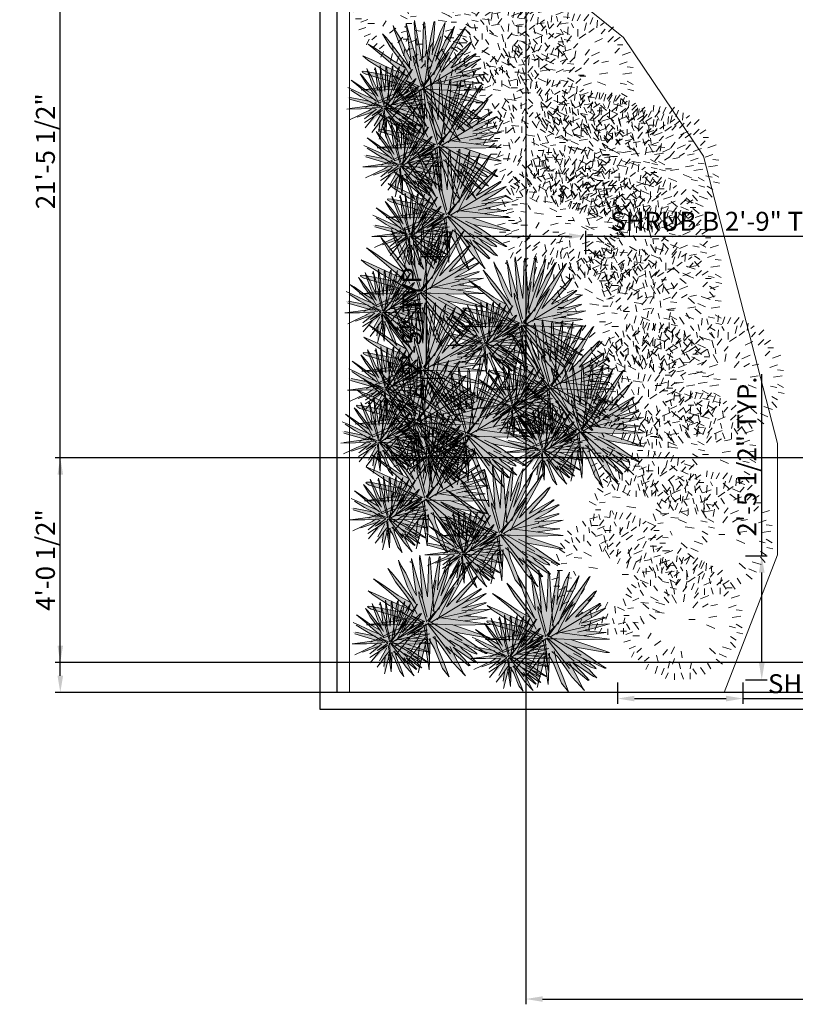
# Model space of a CAD drawing. Units: inches. Extents: x 1239 to 2276906, y 2273 to 321338.
# Tile 1 of 23: x 1239 to 1424, y 2276 to 2510. Entities that reach past the tile are written whole.
import ezdxf

# ---------------------------------------------------------------- set-up
doc = ezdxf.new("R2010")
doc.units = ezdxf.units.IN
for name, color, linetype, lineweight in [('A-ANNO-DIMS', 2, 'Continuous', 18), ('C-PROP', 7, 'Continuous', 25), ('L-PLNT', 94, 'Continuous', 13)]:
    doc.layers.add(name, color=color, linetype=linetype, lineweight=lineweight)
doc.styles.get("Standard").update_dxf_attribs({"font": 'arial.ttf'})
doc.dimstyles.new('ISO-25', dxfattribs={"dimtxt": 4.5, "dimasz": 4, "dimexe": 1.25, "dimexo": 0.625, "dimtad": 1, "dimdec": 1, "dimlunit": 3, "dimtxsty": 'Standard', "dimcen": 2.5, "dimadec": 0, "dimazin": 0, "dimtfac": 1, "dimtdec": 1, "dimtmove": 0, "dimatfit": 3, "dimfxl": 1, "dimarcsym": 0})

# ---------------------------------------------------------------- blocks, each defined once
blk = doc.blocks.new('A$C20C17E7E')
for p, q in [((1.899, 5.117), (1.929, 5.423)), ((2.205, 5.147), (2.144, 5.393)), ((2.635, 5.271), (2.665, 5.546)), ((2.849, 5.179), (2.941, 5.485)), ((3.063, 5.179), (3.217, 5.455)), ((3.37, 5.179), (3.584, 5.455)), ((3.646, 5.025), (3.768, 5.332)), ((1.195, 4.597), (1.134, 4.871)), ((1.562, 4.871), (1.409, 5.086)), ((1.807, 4.871), (1.746, 5.147)), ((2.174, 4.903), (2.359, 5.147)), ((2.635, 4.565), (2.665, 4.903)), ((2.91, 4.871), (2.819, 5.056)), ((3.401, 4.749), (3.492, 5.086)), ((3.952, 4.871), (3.983, 5.21)), ((4.105, 4.964), (4.259, 5.086)), ((4.472, 4.688), (4.687, 4.903)), ((0.919, 4.474), (0.735, 4.658)), ((1.47, 4.198), (1.47, 4.474)), ((1.716, 4.565), (1.685, 4.81)), ((1.991, 4.443), (1.807, 4.627)), ((2.45, 4.565), (2.328, 4.81)), ((2.45, 4.106), (2.359, 4.443)), ((2.604, 4.228), (2.819, 4.504)), ((3.095, 4.474), (3.095, 4.81)), ((3.156, 4.382), (3.462, 4.597)), ((3.584, 4.658), (3.829, 4.841)), ((4.135, 4.597), (4.32, 4.81)), ((4.442, 4.228), (4.687, 4.474)), ((4.717, 4.259), (4.993, 4.443)), ((0.613, 3.861), (0.428, 4.106)), ((0.827, 4.106), (0.613, 4.259)), ((0.98, 4.137), (0.919, 4.352)), ((1.164, 3.77), (1.01, 4.014)), ((1.286, 4.137), (1.102, 4.352)), ((1.777, 3.983), (1.623, 4.198)), ((2.267, 3.739), (2.174, 4.045)), ((2.543, 3.831), (2.513, 4.076)), ((2.91, 3.953), (3.095, 4.167)), ((3.86, 4.228), (4.196, 4.382)), ((4.871, 4.106), (5.117, 4.106)), ((0.367, 3.31), (0.244, 3.616)), ((0.613, 3.677), (0.367, 3.831)), ((0.949, 3.646), (0.674, 3.524)), ((1.807, 3.524), (1.47, 3.707)), ((2.635, 3.431), (2.42, 3.8)), ((2.941, 3.494), (3.002, 3.831)), ((3.431, 3.646), (3.614, 3.892)), ((3.707, 3.616), (4.074, 3.77)), ((4.748, 3.739), (4.963, 3.953)), ((5.086, 3.646), (5.453, 3.77)), ((0.306, 3.095), (0, 3.249)), ((0.704, 3.218), (0.459, 3.188)), ((1.378, 3.431), (1.041, 3.463)), ((3.37, 3.218), (3.584, 3.494)), ((3.799, 3.249), (4.044, 3.401)), ((4.166, 3.31), (4.472, 3.37)), ((4.963, 3.218), (5.3, 3.34)), ((5.3, 3.125), (5.575, 3.095)), ((0.52, 2.88), (0.276, 2.88)), ((1.102, 2.666), (1.01, 2.849)), ((2.083, 2.973), (1.685, 3.034)), ((3.186, 2.697), (3.462, 2.697)), ((4.074, 2.788), (4.442, 2.849)), ((5.117, 2.788), (5.514, 2.849)), ((0.367, 2.574), (0.03, 2.482)), ((0.919, 2.543), (0.674, 2.574)), ((3.983, 2.452), (4.35, 2.298)), ((4.993, 2.391), (5.269, 2.33)), ((5.3, 2.482), (5.575, 2.33)), ((0.398, 2.176), (0.122, 2.176)), ((0.582, 1.778), (0.276, 1.685)), ((0.674, 2.145), (0.367, 2.022)), ((0.98, 1.961), (0.674, 1.961)), ((1.501, 2.084), (1.347, 1.839)), ((5.056, 1.931), (5.3, 1.778)), ((5.331, 2.115), (5.607, 2.054)), ((0.796, 1.502), (0.52, 1.379)), ((1.071, 1.409), (0.858, 1.226)), ((1.929, 1.748), (1.653, 1.533)), ((2.237, 1.348), (2.022, 1.103)), ((2.543, 1.472), (2.389, 1.164)), ((4.105, 1.409), (4.381, 1.164)), ((4.687, 1.472), (5.086, 1.348)), ((5.056, 1.685), (5.269, 1.44)), ((0.735, 1.257), (0.613, 1.012)), ((1.102, 1.073), (0.919, 0.888)), ((1.409, 1.012), (1.195, 0.827)), ((1.746, 1.103), (1.807, 0.797)), ((2.543, 0.951), (2.45, 0.705)), ((2.849, 1.287), (2.88, 0.981)), ((4.411, 0.92), (4.687, 0.705)), ((4.535, 1.164), (4.871, 1.012)), ((1.378, 0.705), (1.256, 0.46)), ((1.777, 0.614), (1.685, 0.276)), ((2.083, 0.521), (1.961, 0.215)), ((2.328, 0.827), (2.267, 0.521)), ((2.757, 0.736), (2.819, 0.491)), ((3.308, 0.766), (3.247, 0.491)), ((3.37, 0.491), (3.523, 0.245)), ((3.707, 0.552), (3.922, 0.245)), ((4.013, 0.736), (4.166, 0.491)), ((2.267, 0.306), (2.144, 0.062)), ((2.543, 0.276), (2.543, 0)), ((2.849, 0.306), (2.941, 0.03)), ((3.247, 0.306), (3.247, 0.03))]:
    blk.add_line(p, q)
blk = doc.blocks.new('A$C545C060E')
h = blk.add_hatch(color=256)
h.set_gradient(color1=(31, 127, 0), color2=(45, 179, 0), one_color=1, tint=0.35, name='INVSPHERICAL')
h.paths.add_polyline_path([(0.529, 2.393), (0.645, 2.304), (1.889, 1.967), (0.489, 1.77), (1.843, 1.787), (1.618, 1.643), (0.635, 1.178), (1.063, 1.326), (1.966, 1.643), (1.461, 1.231), (1.869, 1.417), (2.379, 1.664), (2.177, 1.5), (1.446, 1.03), (1.981, 1.358), (1.481, 0.744), (2.376, 1.553), (1.986, 0.848), (2.48, 1.336), (1.85, 0.496), (2.266, 0.842), (2.223, 0.533), (2.243, 0.142), (2.487, 1.093), (2.615, 0.257), (2.655, 1.214), (3.074, 0.284), (3.303, 0), (2.908, 1.003), (2.846, 1.271), (2.929, 1.199), (3.853, 0.038), (3.428, 0.832), (3.973, 0.376), (4.009, 0.393), (3.432, 1.008), (3.923, 0.676), (4.175, 0.507), (4.274, 0.474), (4.155, 0.583), (4.009, 0.757), (3.765, 0.932), (3.662, 1.051), (4.067, 0.828), (4.243, 0.779), (4.238, 0.801), (3.802, 1.133), (4.534, 0.795), (4.591, 0.795), (4.42, 0.899), (4.103, 1.12), (3.786, 1.34), (3.464, 1.533), (3.968, 1.441), (4.415, 1.362), (4.571, 1.335), (4.695, 1.33), (3.997, 1.572), (3.423, 1.771), (4.695, 1.782), (3.833, 1.912), (4.591, 2.011), (3.836, 2.079), (4.706, 2.305), (3.951, 2.263), (4.55, 2.506), (4.555, 2.528), (4.493, 2.517), (3.734, 2.332), (4.197, 2.577), (4.56, 2.833), (3.786, 2.523), (4.363, 2.959), (4.394, 2.997), (4.363, 2.997), (3.558, 2.528), (3.549, 2.536), (4.087, 3.155), (4.254, 3.422), (4.191, 3.389), (3.209, 2.381), (4.046, 3.912), (3.999, 3.874), (3.09, 2.626), (3.547, 3.58), (3.666, 3.934), (3.35, 3.438), (3.017, 2.752), (3.225, 3.411), (3.345, 4.064), (3.243, 3.868), (3.184, 3.754), (2.919, 3.073), (2.986, 3.83), (2.991, 4.097), (2.96, 4.075), (2.742, 2.981), (2.732, 2.92), (2.659, 4.026), (2.633, 4.092), (2.612, 4.005), (2.56, 2.719), (2.3, 4.135), (2.382, 2.743), (2.025, 4.026), (2.02, 3.934), (1.968, 3.917), (2.046, 3.874), (2.185, 2.776), (1.976, 3.197), (1.829, 3.524), (1.673, 3.773), (1.577, 3.963), (1.613, 3.821), (1.751, 3.44), (1.89, 3.059), (2.192, 2.446), (1.345, 3.551), (1.215, 3.683), (1.481, 3.234), (2.006, 2.515), (1.567, 2.769), (0.983, 3.176), (0.731, 3.334), (1.255, 2.901), (1.969, 2.294), (0.912, 2.769), (0.549, 2.927), (1.687, 2.199), (0.675, 2.399), (0.554, 2.409)])
h = blk.add_hatch(color=256)
h.set_gradient(color1=(31, 127, 0), color2=(55, 219, 0), one_color=1, tint=0.43, name='SPHERICAL')
h.paths.add_polyline_path([(3.023, 2.188), (3.114, 2.362), (3.471, 3.049), (3.33, 2.866), (2.618, 1.891), (2.679, 1.855), (2.94, 2.013)])
h = blk.add_hatch(color=256)
h.set_gradient(color1=(31, 127, 0), color2=(45, 179, 0), one_color=1, tint=0.35, name='INVSPHERICAL')
h.paths.add_polyline_path([(0.025, 1.517), (0.098, 1.461), (0.877, 1.25), (0, 1.126), (0.848, 1.137), (0.707, 1.047), (0.092, 0.756), (0.36, 0.848), (0.925, 1.047), (0.609, 0.789), (0.865, 0.905), (1.184, 1.06), (1.058, 0.958), (0.6, 0.663), (0.935, 0.868), (0.622, 0.484), (1.182, 0.99), (0.938, 0.549), (1.247, 0.855), (0.853, 0.328), (1.113, 0.545), (1.086, 0.352), (1.099, 0.106), (1.252, 0.703), (1.332, 0.179), (1.357, 0.779), (1.62, 0.195), (1.763, 0.018), (1.515, 0.646), (1.477, 0.814), (1.529, 0.769), (2.108, 0.042), (1.841, 0.539), (2.183, 0.253), (2.206, 0.264), (1.844, 0.649), (2.152, 0.441), (2.31, 0.335), (2.371, 0.315), (2.297, 0.383), (2.206, 0.492), (2.053, 0.602), (1.988, 0.676), (2.242, 0.537), (2.352, 0.506), (2.349, 0.52), (2.076, 0.728), (2.534, 0.516), (2.57, 0.516), (2.463, 0.581), (2.264, 0.719), (2.066, 0.857), (1.864, 0.978), (2.18, 0.921), (2.46, 0.871), (2.557, 0.854), (2.636, 0.851), (2.198, 1.003), (1.839, 1.127), (2.636, 1.134), (2.095, 1.216), (2.57, 1.277), (2.097, 1.32), (2.642, 1.462), (2.169, 1.435), (2.544, 1.588), (2.548, 1.602), (2.509, 1.595), (2.033, 1.479), (2.323, 1.632), (2.551, 1.793), (2.066, 1.598), (2.427, 1.871), (2.447, 1.895), (2.427, 1.895), (1.923, 1.602), (1.917, 1.606), (2.255, 1.994), (2.359, 2.161), (2.32, 2.141), (1.704, 1.509), (2.229, 2.469), (2.199, 2.445), (1.63, 1.663), (1.916, 2.26), (1.991, 2.482), (1.792, 2.172), (1.584, 1.741), (1.714, 2.155), (1.789, 2.564), (1.726, 2.441), (1.688, 2.369), (1.522, 1.943), (1.565, 2.417), (1.568, 2.584), (1.548, 2.571), (1.412, 1.885), (1.405, 1.847), (1.36, 2.54), (1.343, 2.581), (1.33, 2.526), (1.298, 1.721), (1.135, 2.608), (1.186, 1.736), (0.962, 2.54), (0.959, 2.482), (0.927, 2.472), (0.976, 2.445), (1.063, 1.757), (0.932, 2.02), (0.84, 2.226), (0.742, 2.381), (0.682, 2.501), (0.704, 2.411), (0.791, 2.173), (0.878, 1.934), (1.067, 1.55), (0.537, 2.242), (0.455, 2.325), (0.622, 2.044), (0.951, 1.593), (0.676, 1.752), (0.31, 2.007), (0.152, 2.107), (0.48, 1.835), (0.927, 1.455), (0.265, 1.752), (0.038, 1.851), (0.751, 1.395), (0.117, 1.52), (0.041, 1.527)])
h = blk.add_hatch(color=256)
h.set_gradient(color1=(31, 127, 0), color2=(55, 219, 0), one_color=1, tint=0.43, name='SPHERICAL')
h.paths.add_polyline_path([(1.334, 1.202), (1.372, 1.18), (1.536, 1.279), (1.588, 1.388), (1.645, 1.497), (1.868, 1.928), (1.78, 1.813)])
for p, q in [((2.02, 3.934, -52.769), (2.025, 4.026, -52.769)), ((2.025, 4.026, -52.769), (2.389, 2.719, -52.769)), ((2.295, 4.037, -52.769), (2.3, 4.135, -52.769)), ((2.389, 2.643, -52.769), (2.295, 4.037, -52.769)), ((2.3, 4.135, -52.769), (2.534, 2.893, -52.769)), ((2.612, 4.005, -52.769), (2.633, 4.092, -52.769)), ((2.633, 4.092, -52.769), (2.659, 4.026, -52.769)), ((2.659, 4.026, -52.769), (2.732, 2.92, -52.769)), ((2.945, 4.01, -52.769), (2.96, 4.075, -52.769)), ((2.96, 4.075, -52.769), (2.991, 4.097, -52.769)), ((2.991, 4.097, -52.769), (2.986, 3.83, -52.769)), ((3.345, 4.064, -52.769), (3.225, 3.411, -52.769)), ((3.303, 3.983, -52.769), (3.345, 4.064, -52.769)), ((1.215, 3.683, -52.769), (1.481, 3.234, -52.769)), ((1.345, 3.551, -52.769), (1.215, 3.683, -52.769)), ((1.577, 3.963, -52.769), (1.613, 3.821, -52.769)), ((1.673, 3.773, -52.769), (1.577, 3.963, -52.769)), ((1.613, 3.821, -52.769), (1.89, 3.059, -52.769)), ((1.829, 3.524, -52.769), (1.673, 3.773, -52.769)), ((1.968, 3.917, -52.769), (2.02, 3.934, -52.769)), ((2.046, 3.874, -52.769), (1.968, 3.917, -52.769)), ((2.103, 3.378, -52.769), (2.046, 3.874, -52.769)), ((2.591, 3.329, -52.769), (2.612, 4.005, -52.769)), ((2.742, 2.981, -52.769), (2.945, 4.01, -52.769)), ((2.986, 3.83, -52.769), (2.908, 2.964, -52.769)), ((3.095, 3.498, -52.769), (3.184, 3.754, -52.769)), ((3.184, 3.754, -52.769), (3.303, 3.983, -52.769)), ((3.428, 3.553, -52.769), (3.666, 3.934, -52.769)), ((3.508, 3.479, -52.769), (3.625, 3.884, -52.769)), ((3.666, 3.934, -52.769), (3.547, 3.58, -52.769)), ((3.558, 3.269, -52.769), (3.999, 3.874, -52.769)), ((4.046, 3.912, -52.769), (3.635, 3.155, -52.769)), ((3.999, 3.874, -52.769), (4.046, 3.912, -52.769)), ((1.602, 3.229, -52.769), (1.345, 3.551, -52.769)), ((1.976, 3.197, -52.769), (1.829, 3.524, -52.769)), ((2.186, 2.773, -52.769), (2.103, 3.378, -52.769)), ((3.198, 3.588, -52.769), (2.75, 2.248, -52.769)), ((2.919, 3.073, -52.769), (3.095, 3.498, -52.769)), ((3.225, 3.411, -52.769), (3.017, 2.752, -52.769)), ((3.547, 3.58, -52.769), (3.085, 2.626, -52.769)), ((3.298, 3.329, -52.769), (3.35, 3.438, -52.769)), ((3.35, 3.438, -52.769), (3.428, 3.553, -52.769)), ((3.771, 2.975, -52.769), (4.191, 3.389, -52.769)), ((4.254, 3.422, -52.769), (4.087, 3.155, -52.769)), ((4.191, 3.389, -52.769), (4.254, 3.422, -52.769)), ((0.731, 3.334, -52.769), (1.255, 2.901, -52.769)), ((0.983, 3.176, -52.769), (0.731, 3.334, -52.769)), ((1.567, 2.769, -52.769), (0.983, 3.176, -52.769)), ((1.481, 3.234, -52.769), (1.819, 2.785, -52.769)), ((2.157, 2.505, -52.769), (1.602, 3.229, -52.769)), ((1.89, 3.059, -52.769), (2.192, 2.446, -52.769)), ((2.102, 2.927, -52.769), (1.976, 3.197, -52.769)), ((2.56, 2.719, -52.769), (2.591, 3.329, -52.769)), ((2.849, 3.284, -52.769), (2.65, 1.996, -52.769)), ((3.017, 2.752, -52.769), (3.298, 3.329, -52.769)), ((3.09, 2.626, -52.769), (3.558, 3.269, -52.769)), ((3.471, 3.049, -52.769), (3.114, 2.362, -52.769)), ((3.635, 3.155, -52.769), (3.209, 2.381, -52.769)), ((3.33, 2.866, -52.769), (3.471, 3.049, -52.769)), ((4.087, 3.155, -52.769), (3.542, 2.528, -52.769)), ((0.549, 2.927, -52.769), (0.72, 2.785, -52.769)), ((0.912, 2.769, -52.769), (0.549, 2.927, -52.769)), ((0.72, 2.785, -52.769), (1.27, 2.43, -52.769)), ((1.522, 2.483, -52.769), (0.912, 2.769, -52.769)), ((1.255, 2.901, -52.769), (1.653, 2.552, -52.769)), ((2.006, 2.515, -52.769), (1.567, 2.769, -52.769)), ((1.819, 2.785, -52.769), (2.016, 2.494, -52.769)), ((2.192, 2.764, -52.769), (2.102, 2.927, -52.769)), ((2.269, 2.899, -52.769), (2.394, 2.654, -52.769)), ((2.279, 2.724, -52.769), (2.269, 2.899, -52.769)), ((2.539, 1.864, -52.769), (2.279, 2.724, -52.769)), ((2.534, 2.893, -52.769), (2.56, 2.719, -52.769)), ((2.6, 1.866, -52.769), (3.33, 2.866, -52.769)), ((2.732, 2.92, -52.769), (2.783, 2.212, -52.769)), ((3.209, 2.381, -52.769), (3.771, 2.975, -52.769)), ((3.558, 2.528, -52.769), (4.327, 2.975, -52.769)), ((4.363, 2.959, -52.769), (3.786, 2.523, -52.769)), ((3.797, 2.528, -52.769), (4.191, 2.692, -52.769)), ((4.191, 2.692, -52.769), (4.514, 2.822, -52.769)), ((4.56, 2.833, -52.769), (4.197, 2.577, -52.769)), ((4.327, 2.975, -52.769), (4.363, 2.997, -52.769)), ((4.394, 2.997, -52.769), (4.363, 2.959, -52.769)), ((4.363, 2.997, -52.769), (4.394, 2.997, -52.769)), ((4.514, 2.822, -52.769), (4.56, 2.833, -52.769)), ((0.554, 2.409, -52.769), (0.529, 2.393, -52.769)), ((0.529, 2.393, -52.769), (0.539, 2.367, -52.769)), ((0.539, 2.367, -52.769), (0.645, 2.304, -52.769)), ((0.675, 2.399, -52.769), (0.554, 2.409, -52.769)), ((1.32, 2.272, -52.769), (0.675, 2.399, -52.769)), ((0.682, 2.501), (0.704, 2.411)), ((0.742, 2.381), (0.682, 2.501)), ((0.704, 2.411), (0.878, 1.934)), ((0.84, 2.226), (0.742, 2.381)), ((0.927, 2.472), (0.959, 2.482)), ((0.976, 2.445), (0.927, 2.472)), ((0.959, 2.482), (0.962, 2.54)), ((0.962, 2.54), (1.19, 1.721)), ((1.011, 2.134), (0.976, 2.445)), ((1.132, 2.547), (1.135, 2.608)), ((1.19, 1.673), (1.132, 2.547)), ((1.135, 2.608), (1.281, 1.83)), ((1.27, 2.43, -52.769), (1.764, 2.156, -52.769)), ((1.317, 2.103), (1.33, 2.526)), ((1.33, 2.526), (1.343, 2.581)), ((1.343, 2.581), (1.36, 2.54)), ((1.36, 2.54), (1.405, 1.847)), ((1.412, 1.885), (1.539, 2.53)), ((1.565, 2.417), (1.516, 1.875)), ((2.046, 2.261, -52.769), (1.522, 2.483, -52.769)), ((1.539, 2.53), (1.548, 2.571)), ((1.548, 2.571), (1.568, 2.584)), ((1.568, 2.584), (1.565, 2.417)), ((1.633, 2.209), (1.688, 2.369)), ((1.653, 2.552, -52.769), (2.087, 2.198, -52.769)), ((1.688, 2.369), (1.763, 2.513)), ((1.789, 2.564), (1.714, 2.155)), ((1.763, 2.513), (1.789, 2.564)), ((1.841, 2.243), (1.991, 2.482)), ((1.891, 2.197), (1.965, 2.451)), ((1.991, 2.482), (1.916, 2.26)), ((1.923, 2.066), (2.199, 2.445)), ((2.229, 2.469), (1.971, 1.994)), ((2.016, 2.494, -52.769), (2.208, 2.129, -52.769)), ((2.199, 2.445), (2.229, 2.469)), ((2.394, 2.654, -52.769), (2.55, 2.027, -52.769)), ((3.786, 2.523, -52.769), (2.674, 1.853, -52.769)), ((3.085, 2.626, -52.769), (2.955, 2.288, -52.769)), ((3.114, 2.362, -52.769), (3.023, 2.188, -52.769)), ((3.734, 2.332, -52.769), (4.493, 2.517, -52.769)), ((3.848, 2.381, -52.769), (3.734, 2.332, -52.769)), ((4.197, 2.577, -52.769), (3.848, 2.381, -52.769)), ((4.55, 2.506, -52.769), (3.854, 2.223, -52.769)), ((4.493, 2.517, -52.769), (4.555, 2.528, -52.769)), ((4.555, 2.528, -52.769), (4.55, 2.506, -52.769)), ((0.152, 2.107), (0.48, 1.835)), ((0.31, 2.007), (0.152, 2.107)), ((0.676, 1.752), (0.31, 2.007)), ((0.455, 2.325), (0.622, 2.044)), ((0.537, 2.242), (0.455, 2.325)), ((0.698, 2.04), (0.537, 2.242)), ((0.622, 2.044), (0.834, 1.762)), ((0.645, 2.304, -52.769), (1.734, 1.992, -52.769)), ((1.045, 1.587), (0.698, 2.04)), ((0.932, 2.02), (0.84, 2.226)), ((1.011, 1.851), (0.932, 2.02)), ((1.063, 1.755), (1.011, 2.134)), ((1.298, 1.721), (1.317, 2.103)), ((1.769, 2.182, -52.769), (1.32, 2.272, -52.769)), ((1.479, 2.075), (1.354, 1.268)), ((1.697, 2.266), (1.416, 1.426)), ((1.522, 1.943), (1.633, 2.209)), ((1.714, 2.155), (1.584, 1.741)), ((1.584, 1.741), (1.76, 2.103)), ((1.916, 2.26), (1.627, 1.663)), ((1.63, 1.663), (1.923, 2.066)), ((1.76, 2.103), (1.792, 2.172)), ((1.764, 2.156, -52.769), (2.182, 1.902, -52.769)), ((1.792, 2.172), (1.841, 2.243)), ((2.009, 2.092, -52.769), (2.476, 1.885, -52.769)), ((2.425, 1.814, -52.769), (2.009, 2.092, -52.769)), ((2.056, 1.881), (2.32, 2.141)), ((2.359, 2.161), (2.255, 1.994)), ((2.32, 2.141), (2.359, 2.161)), ((2.565, 1.907, -52.769), (2.84, 2.229, -52.769)), ((2.84, 2.229, -52.769), (2.606, 1.885, -52.769)), ((3.878, 2.205, -52.769), (2.857, 1.97, -52.769)), ((3.023, 2.188, -52.769), (2.907, 1.944, -52.769)), ((4.228, 2.169, -52.769), (3.61, 2.027, -52.769)), ((3.734, 2.25, -52.769), (4.301, 2.283, -52.769)), ((3.807, 2.082, -52.769), (4.264, 2.038, -52.769)), ((4.591, 2.011, -52.769), (3.833, 1.912, -52.769)), ((3.886, 2.102, -52.769), (3.98, 2.099, -52.769)), ((3.949, 2.282, -52.769), (4.001, 2.285, -52.769)), ((3.98, 2.099, -52.769), (4.025, 2.091, -52.769)), ((4.001, 2.285, -52.769), (4.042, 2.282, -52.769)), ((4.706, 2.305, -52.769), (4.228, 2.169, -52.769)), ((4.264, 2.038, -52.769), (4.534, 2.016, -52.769)), ((4.301, 2.283, -52.769), (4.706, 2.305, -52.769)), ((4.534, 2.016, -52.769), (4.591, 2.011, -52.769)), ((0.265, 1.752), (0.038, 1.851)), ((0.145, 1.762), (0.49, 1.54)), ((0.647, 1.573), (0.265, 1.752)), ((0.48, 1.835), (0.729, 1.617)), ((0.64, 1.791, -52.769), (0.489, 1.77, -52.769)), ((0.489, 1.77, -52.769), (1.275, 1.775, -52.769)), ((1.068, 1.844, -52.769), (0.64, 1.791, -52.769)), ((0.951, 1.593), (0.676, 1.752)), ((0.834, 1.762), (0.957, 1.58)), ((0.878, 1.934), (1.067, 1.55)), ((1.067, 1.749), (1.011, 1.851)), ((1.981, 1.981, -52.769), (1.068, 1.844, -52.769)), ((1.115, 1.834), (1.194, 1.68)), ((1.122, 1.724), (1.115, 1.834)), ((1.285, 1.185), (1.122, 1.724)), ((1.194, 1.68), (1.291, 1.288)), ((1.275, 1.775, -52.769), (2.051, 1.791, -52.769)), ((1.281, 1.83), (1.298, 1.721)), ((1.323, 1.186), (1.78, 1.813)), ((1.405, 1.847), (1.438, 1.404)), ((1.678, 1.675, -52.769), (1.618, 1.643, -52.769)), ((1.868, 1.928), (1.645, 1.497)), ((1.865, 1.801, -52.769), (1.678, 1.675, -52.769)), ((1.971, 1.994), (1.704, 1.509)), ((1.704, 1.509), (2.056, 1.881)), ((1.734, 1.992, -52.769), (2.006, 1.949, -52.769)), ((1.78, 1.813), (1.868, 1.928)), ((1.869, 1.417, -52.769), (2.425, 1.814, -52.769)), ((2.456, 1.716, -52.769), (1.869, 1.417, -52.769)), ((1.87, 1.874, -52.769), (2.276, 1.84, -52.769)), ((2.255, 1.994), (1.913, 1.602)), ((1.923, 1.602), (2.404, 1.881)), ((1.966, 1.643, -52.769), (2.107, 1.77, -52.769)), ((2.427, 1.871), (2.066, 1.598)), ((2.072, 1.602), (2.32, 1.704)), ((2.32, 1.704), (2.522, 1.786)), ((2.551, 1.793), (2.323, 1.632)), ((2.404, 1.881), (2.427, 1.895)), ((2.447, 1.895), (2.427, 1.871)), ((2.427, 1.895), (2.447, 1.895)), ((2.617, 0.725, -52.769), (2.456, 1.716, -52.769)), ((2.513, 1.809, -52.769), (2.617, 0.725, -52.769)), ((2.522, 1.786), (2.551, 1.793)), ((2.913, 1.793, -52.769), (2.555, 1.798, -52.769)), ((3.347, 0.787, -52.769), (2.559, 1.822, -52.769)), ((3.504, 1.039, -52.769), (2.584, 1.831, -52.769)), ((3.737, 1.239, -52.769), (2.617, 1.892, -52.769)), ((3.672, 1.76, -52.769), (2.913, 1.793, -52.769)), ((3.516, 1.945, -52.769), (3.028, 2.005, -52.769)), ((3.422, 1.766, -52.769), (4.571, 1.379, -52.769)), ((4.701, 1.782, -52.769), (3.516, 1.945, -52.769)), ((4.695, 1.782, -52.769), (3.672, 1.76, -52.769)), ((0.098, 1.461), (0.78, 1.265)), ((0.521, 1.441), (0.117, 1.52)), ((0.49, 1.54), (0.799, 1.368)), ((0.802, 1.385), (0.521, 1.441)), ((1.048, 1.379, -52.769), (0.635, 1.178, -52.769)), ((0.976, 1.434), (0.647, 1.573)), ((0.729, 1.617), (1.001, 1.395)), ((0.799, 1.368), (1.061, 1.209)), ((0.957, 1.58), (1.077, 1.352)), ((1.345, 1.521, -52.769), (1.048, 1.379, -52.769)), ((1.063, 1.326, -52.769), (1.608, 1.516, -52.769)), ((1.301, 1.212), (1.473, 1.414)), ((1.473, 1.414), (1.327, 1.199)), ((1.618, 1.643, -52.769), (1.345, 1.521, -52.769)), ((2.066, 1.598), (1.369, 1.178)), ((1.446, 1.03, -52.769), (2.177, 1.5, -52.769)), ((1.966, 1.643, -52.769), (1.461, 1.231, -52.769)), ((1.981, 1.358, -52.769), (1.481, 0.744, -52.769)), ((2.123, 1.399), (1.484, 1.252)), ((1.588, 1.388), (1.515, 1.235)), ((1.627, 1.663), (1.545, 1.451)), ((1.645, 1.497), (1.588, 1.388)), ((1.608, 1.516, -52.769), (1.966, 1.643, -52.769)), ((2.343, 1.376), (1.955, 1.288)), ((1.986, 0.848, -52.769), (2.376, 1.553, -52.769)), ((2.033, 1.479), (2.509, 1.595)), ((2.105, 1.509), (2.033, 1.479)), ((2.033, 1.427), (2.388, 1.448)), ((2.323, 1.632), (2.105, 1.509)), ((2.544, 1.588), (2.108, 1.41)), ((2.168, 1.447), (2.2, 1.449)), ((2.177, 1.5, -52.769), (2.379, 1.664, -52.769)), ((2.2, 1.449), (2.226, 1.447)), ((2.642, 1.462), (2.343, 1.376)), ((2.388, 1.448), (2.642, 1.462)), ((2.509, 1.595), (2.548, 1.602)), ((2.548, 1.602), (2.544, 1.588)), ((2.929, 1.199, -52.769), (2.742, 1.362, -52.769)), ((2.819, 1.39, -52.769), (2.908, 1.003, -52.769)), ((3.443, 1.537, -52.769), (3.178, 1.657, -52.769)), ((3.677, 1.493, -52.769), (3.443, 1.537, -52.769)), ((3.448, 1.542, -52.769), (3.786, 1.34, -52.769)), ((4.259, 1.39, -52.769), (3.677, 1.493, -52.769)), ((3.786, 1.34, -52.769), (4.42, 0.899, -52.769)), ((4.571, 1.335, -52.769), (4.259, 1.39, -52.769)), ((4.571, 1.379, -52.769), (4.695, 1.33, -52.769)), ((0, 1.126), (0.493, 1.13)), ((0.363, 1.173), (0.095, 1.14)), ((0.935, 1.259), (0.363, 1.173)), ((0.493, 1.13), (0.979, 1.14)), ((0.707, 1.047), (0.537, 0.971)), ((0.925, 1.047), (0.609, 0.789)), ((0.701, 0.967), (0.925, 1.047)), ((0.745, 1.067), (0.707, 1.047)), ((0.862, 1.146), (0.745, 1.067)), ((0.78, 1.265), (0.951, 1.239)), ((0.865, 0.905), (1.213, 1.154)), ((1.232, 1.093), (0.865, 0.905)), ((0.866, 1.192), (1.12, 1.17)), ((0.925, 1.047), (1.014, 1.126)), ((0.952, 1.328), (1.245, 1.199)), ((1.213, 1.154), (0.952, 1.328)), ((1.058, 0.958), (1.184, 1.06)), ((1.333, 0.472), (1.232, 1.093)), ((1.268, 1.151), (1.333, 0.472)), ((1.519, 1.141), (1.294, 1.144)), ((1.791, 0.511), (1.297, 1.159)), ((1.889, 0.669), (1.312, 1.165)), ((2.035, 0.794), (1.333, 1.203)), ((1.994, 1.12), (1.519, 1.141)), ((1.897, 1.236), (1.591, 1.274)), ((1.851, 0.98), (1.685, 1.056)), ((1.838, 1.124), (2.557, 0.881)), ((1.85, 0.496, -52.769), (2.313, 1.109, -52.769)), ((2.639, 1.134), (1.897, 1.236)), ((2.636, 1.134), (1.994, 1.12)), ((2.079, 1.322), (2.365, 1.294)), ((2.57, 1.277), (2.095, 1.216)), ((2.128, 1.335), (2.187, 1.333)), ((2.187, 1.333), (2.215, 1.328)), ((2.308, 1.151, -52.769), (2.223, 0.533, -52.769)), ((2.243, 0.142, -52.769), (2.485, 1.067, -52.769)), ((2.313, 1.109, -52.769), (2.48, 1.336, -52.769)), ((2.365, 1.294), (2.534, 1.281)), ((2.617, 0.245, -52.769), (2.471, 1.199, -52.769)), ((2.485, 1.067, -52.769), (2.5, 1.22, -52.769)), ((2.534, 1.281), (2.57, 1.277)), ((2.799, 0.97, -52.769), (2.606, 1.297, -52.769)), ((2.658, 1.308, -52.769), (2.617, 0.245, -52.769)), ((3.427, 0.496, -52.769), (2.929, 1.199, -52.769)), ((3.973, 0.376, -52.769), (3.204, 1.019, -52.769)), ((3.62, 1.074, -52.769), (3.313, 1.248, -52.769)), ((3.324, 1.03, -52.769), (3.599, 0.507, -52.769)), ((3.687, 0.839, -52.769), (3.432, 1.008, -52.769)), ((3.432, 1.008, -52.769), (3.786, 0.643, -52.769)), ((3.802, 1.133, -52.769), (3.479, 1.292, -52.769)), ((4.067, 0.828, -52.769), (3.62, 1.074, -52.769)), ((3.656, 1.057, -52.769), (3.765, 0.932, -52.769)), ((4.243, 0.932, -52.769), (3.802, 1.133, -52.769)), ((3.802, 1.128, -52.769), (4.176, 0.856, -52.769)), ((4.695, 1.33, -52.769), (4.571, 1.335, -52.769)), ((0.351, 0.881), (0.092, 0.756)), ((0.537, 0.971), (0.351, 0.881)), ((0.36, 0.848), (0.701, 0.967)), ((0.6, 0.663), (1.058, 0.958)), ((0.935, 0.868), (0.622, 0.484)), ((0.853, 0.328), (1.143, 0.713)), ((0.938, 0.549), (1.182, 0.99)), ((1.14, 0.739), (1.086, 0.352)), ((1.099, 0.106), (1.251, 0.686)), ((1.143, 0.713), (1.247, 0.855)), ((1.333, 0.171), (1.242, 0.769)), ((1.251, 0.686), (1.26, 0.782)), ((1.447, 0.625), (1.327, 0.83)), ((1.359, 0.837), (1.333, 0.171)), ((1.529, 0.769), (1.411, 0.871)), ((1.46, 0.888), (1.515, 0.646)), ((1.841, 0.328), (1.529, 0.769)), ((1.962, 0.69), (1.77, 0.799)), ((1.997, 0.953), (1.851, 0.98)), ((1.854, 0.984), (2.066, 0.857)), ((2.076, 0.728), (1.874, 0.827)), ((2.242, 0.537), (1.962, 0.69)), ((1.984, 0.68), (2.053, 0.602)), ((2.362, 0.888), (1.997, 0.953)), ((2.066, 0.857), (2.463, 0.581)), ((2.352, 0.602), (2.076, 0.728)), ((2.076, 0.724), (2.31, 0.554)), ((2.557, 0.854), (2.362, 0.888)), ((2.557, 0.881), (2.636, 0.851)), ((2.636, 0.851), (2.557, 0.854)), ((3.074, 0.284, -52.769), (2.799, 0.97, -52.769)), ((2.908, 1.003, -52.769), (3.111, 0.512, -52.769)), ((4.16, 0.512, -52.769), (3.687, 0.839, -52.769)), ((3.765, 0.932, -52.769), (4.009, 0.757, -52.769)), ((4.009, 0.757, -52.769), (4.155, 0.583, -52.769)), ((4.243, 0.779, -52.769), (4.067, 0.828, -52.769)), ((4.176, 0.856, -52.769), (4.238, 0.801, -52.769)), ((4.238, 0.801, -52.769), (4.243, 0.779, -52.769)), ((4.534, 0.795, -52.769), (4.243, 0.932, -52.769)), ((4.42, 0.899, -52.769), (4.591, 0.795, -52.769)), ((4.591, 0.795, -52.769), (4.534, 0.795, -52.769)), ((1.62, 0.195), (1.447, 0.625)), ((1.515, 0.646), (1.643, 0.339)), ((1.643, 0.339), (1.763, 0.018)), ((2.183, 0.253), (1.701, 0.656)), ((1.776, 0.663), (1.948, 0.335)), ((2.004, 0.543), (1.844, 0.649)), ((1.844, 0.649), (2.066, 0.421)), ((1.948, 0.335), (2.066, 0.1)), ((2.3, 0.339), (2.004, 0.543)), ((2.053, 0.602), (2.206, 0.492)), ((2.066, 0.421), (2.206, 0.264)), ((2.206, 0.492), (2.297, 0.383)), ((2.352, 0.506), (2.242, 0.537)), ((2.297, 0.383), (2.371, 0.315)), ((2.371, 0.315), (2.3, 0.339)), ((2.31, 0.554), (2.349, 0.52)), ((2.349, 0.52), (2.352, 0.506)), ((2.534, 0.516), (2.352, 0.602)), ((2.463, 0.581), (2.57, 0.516)), ((2.57, 0.516), (2.534, 0.516)), ((3.111, 0.512, -52.769), (3.303, 0, -52.769)), ((3.853, 0.038, -52.769), (3.427, 0.496, -52.769)), ((3.599, 0.507, -52.769), (3.786, 0.131, -52.769)), ((3.786, 0.643, -52.769), (4.009, 0.393, -52.769)), ((4.009, 0.393, -52.769), (3.973, 0.376, -52.769)), ((4.155, 0.583, -52.769), (4.274, 0.474, -52.769)), ((4.274, 0.474, -52.769), (4.16, 0.512, -52.769)), ((1.763, 0.018), (1.62, 0.195)), ((2.108, 0.042), (1.841, 0.328)), ((2.066, 0.1), (2.108, 0.042)), ((2.206, 0.264), (2.183, 0.253)), ((3.303, 0, -52.769), (3.074, 0.284, -52.769)), ((3.786, 0.131, -52.769), (3.853, 0.038, -52.769))]:
    blk.add_line(p, q)
blk = doc.blocks.new('t1')
at = {"xscale": 1200, "yscale": 1200, "zscale": 1200}
blk.add_blockref('A$C545C060E', (1649217, 160231), dxfattribs=at)
blk = doc.blocks.new('*D76')
at = {"layer": 'A-ANNO-DIMS', "color": 0, "lineweight": -2, "transparency": 16777216}
for p, q in [((1381.23, 2352.31), (1381.23, 2347.21)), ((1411.06, 2352.31), (1411.06, 2347.21)), ((1385.23, 2348.46), (1407.06, 2348.46)), ((1411.06, 2348.46), (1473.41, 2348.46))]:
    blk.add_line(p, q, dxfattribs=at)
at = {"layer": 'A-ANNO-DIMS', "color": 0, "transparency": 16777216}
for points in [[(1385.23, 2349.13), (1385.23, 2347.79), (1381.23, 2348.46)], [(1407.06, 2349.13), (1407.06, 2347.79), (1411.06, 2348.46)]]:
    blk.add_solid(points, dxfattribs=at)
at = {"layer": 'Defpoints', "color": 0, "transparency": 16777216}
for p in [(1381.23, 2352.93), (1411.06, 2352.93), (1411.06, 2348.46)]:
    blk.add_point(p, dxfattribs=at)
at = {"layer": 'A-ANNO-DIMS', "color": 0, "transparency": 16777216, "insert": (1444.23, 2351.41), "char_height": 4.5, "attachment_point": 5}
blk.add_mtext('SHRUB A 2\'-6" TYP.', dxfattribs=at)
blk = doc.blocks.new('*D77')
at = {"layer": 'A-ANNO-DIMS', "color": 0, "lineweight": -2, "transparency": 16777216}
for p, q in [((1415.53, 2382.44), (1415.53, 2425.68)), ((1411.68, 2382.44), (1416.78, 2382.44)), ((1415.53, 2356.93), (1415.53, 2378.44)), ((1411.68, 2352.93), (1416.78, 2352.93))]:
    blk.add_line(p, q, dxfattribs=at)
at = {"layer": 'A-ANNO-DIMS', "color": 0, "transparency": 16777216}
for points in [[(1414.87, 2378.44), (1416.2, 2378.44), (1415.53, 2382.44)], [(1414.87, 2356.93), (1416.2, 2356.93), (1415.53, 2352.93)]]:
    blk.add_solid(points, dxfattribs=at)
at = {"layer": 'Defpoints', "color": 0, "transparency": 16777216}
for p in [(1411.06, 2382.44), (1415.53, 2382.44), (1411.06, 2352.93)]:
    blk.add_point(p, dxfattribs=at)
at = {"layer": 'A-ANNO-DIMS', "color": 0, "transparency": 16777216, "insert": (1412.58, 2406.06), "char_height": 4.5, "attachment_point": 5, "rotation": 90}
blk.add_mtext('2\'-5 1/2" TYP.', dxfattribs=at)
blk = doc.blocks.new('*D78')
at = {"layer": 'A-ANNO-DIMS', "color": 0, "lineweight": -2, "transparency": 16777216}
for p, q in [((1340.71, 2454.19), (1340.71, 2459.76)), ((1344.71, 2458.51), (1369.67, 2458.51)), ((1373.67, 2454.19), (1373.67, 2459.76)), ((1373.67, 2458.51), (1436.02, 2458.51))]:
    blk.add_line(p, q, dxfattribs=at)
at = {"layer": 'A-ANNO-DIMS', "color": 0, "transparency": 16777216}
for points in [[(1344.71, 2459.18), (1344.71, 2457.84), (1340.71, 2458.51)], [(1369.67, 2459.18), (1369.67, 2457.84), (1373.67, 2458.51)]]:
    blk.add_solid(points, dxfattribs=at)
at = {"layer": 'Defpoints', "color": 0, "transparency": 16777216}
for p in [(1373.67, 2458.51), (1340.71, 2453.57), (1373.67, 2453.57)]:
    blk.add_point(p, dxfattribs=at)
at = {"layer": 'A-ANNO-DIMS', "color": 0, "transparency": 16777216, "insert": (1406.85, 2461.46), "char_height": 4.5, "attachment_point": 5}
blk.add_mtext('SHRUB B 2\'-9" TYP.', dxfattribs=at)
blk = doc.blocks.new('*D79')
at = {"layer": 'A-ANNO-DIMS', "color": 0, "lineweight": -2, "transparency": 16777216}
for p, q in [((1340.08, 2453.57), (1334.51, 2453.57)), ((1335.76, 2428.59), (1335.76, 2449.57)), ((1340.08, 2424.59), (1334.51, 2424.59))]:
    blk.add_line(p, q, dxfattribs=at)
at = {"layer": 'A-ANNO-DIMS', "color": 0, "transparency": 16777216}
for points in [[(1335.09, 2449.57), (1336.43, 2449.57), (1335.76, 2453.57)], [(1335.09, 2428.59), (1336.43, 2428.59), (1335.76, 2424.59)]]:
    blk.add_solid(points, dxfattribs=at)
at = {"layer": 'Defpoints', "color": 0, "transparency": 16777216}
for p in [(1335.76, 2453.57), (1340.71, 2453.57), (1340.71, 2424.59)]:
    blk.add_point(p, dxfattribs=at)
at = {"layer": 'A-ANNO-DIMS', "color": 0, "transparency": 16777216, "insert": (1332.84, 2439.08), "char_height": 4.5, "attachment_point": 5, "rotation": 90}
blk.add_mtext('2\'-5" TYP.', dxfattribs=at)
blk = doc.blocks.new('*D89')
at = {"layer": 'A-ANNO-DIMS', "color": 0, "lineweight": -2, "transparency": 16777216}
for p, q in [((1359.38, 3215.77), (1359.38, 2275.7)), ((1551.38, 3215.77), (1551.38, 2275.7)), ((1363.38, 2276.95), (1547.38, 2276.95))]:
    blk.add_line(p, q, dxfattribs=at)
at = {"layer": 'A-ANNO-DIMS', "color": 0, "transparency": 16777216}
for points in [[(1363.38, 2277.61), (1363.38, 2276.28), (1359.38, 2276.95)], [(1547.38, 2277.61), (1547.38, 2276.28), (1551.38, 2276.95)]]:
    blk.add_solid(points, dxfattribs=at)
at = {"layer": 'Defpoints', "color": 0, "transparency": 16777216}
for p in [(1359.38, 3216.4), (1551.38, 3216.4), (1551.38, 2276.95)]:
    blk.add_point(p, dxfattribs=at)
at = {"layer": 'A-ANNO-DIMS', "color": 0, "transparency": 16777216, "insert": (1455.38, 2279.87), "char_height": 4.5, "attachment_point": 5}
blk.add_mtext('16\'-0"', dxfattribs=at)
blk = doc.blocks.new('*D103')
at = {"layer": 'A-ANNO-DIMS', "color": 0, "lineweight": -2, "transparency": 16777216}
for p, q in [((1539.93, 2607.52), (1247.33, 2607.52)), ((1248.58, 2353.9), (1248.58, 2603.52)), ((1539.93, 2349.9), (1247.33, 2349.9))]:
    blk.add_line(p, q, dxfattribs=at)
at = {"layer": 'A-ANNO-DIMS', "color": 0, "transparency": 16777216}
for points in [[(1247.92, 2603.52), (1249.25, 2603.52), (1248.58, 2607.52)], [(1247.92, 2353.9), (1249.25, 2353.9), (1248.58, 2349.9)]]:
    blk.add_solid(points, dxfattribs=at)
at = {"layer": 'Defpoints', "color": 0, "transparency": 16777216}
for p in [(1248.58, 2607.52), (1540.55, 2607.52), (1540.55, 2349.9)]:
    blk.add_point(p, dxfattribs=at)
at = {"layer": 'A-ANNO-DIMS', "color": 0, "transparency": 16777216, "insert": (1245.63, 2478.71), "char_height": 4.5, "attachment_point": 5, "rotation": 90}
blk.add_mtext('21\'-5 1/2"', dxfattribs=at)
blk = doc.blocks.new('*D118')
at = {"layer": 'A-ANNO-DIMS', "color": 0, "lineweight": -2, "transparency": 16777216}
for p, q in [((1745.95, 2405.77), (1247.33, 2405.77)), ((1248.58, 2361.06), (1248.58, 2401.77)), ((1745.95, 2357.06), (1247.33, 2357.06))]:
    blk.add_line(p, q, dxfattribs=at)
at = {"layer": 'A-ANNO-DIMS', "color": 0, "transparency": 16777216}
for points in [[(1247.92, 2401.77), (1249.25, 2401.77), (1248.58, 2405.77)], [(1247.92, 2361.06), (1249.25, 2361.06), (1248.58, 2357.06)]]:
    blk.add_solid(points, dxfattribs=at)
at = {"layer": 'Defpoints', "color": 0, "transparency": 16777216}
for p in [(1248.58, 2405.77), (1746.57, 2405.77), (1746.57, 2357.06)]:
    blk.add_point(p, dxfattribs=at)
at = {"layer": 'A-ANNO-DIMS', "color": 0, "transparency": 16777216, "insert": (1245.63, 2381.42), "char_height": 4.5, "attachment_point": 5, "rotation": 90}
blk.add_mtext('4\'-0 1/2"', dxfattribs=at)

msp = doc.modelspace()

# ---------------------------------------------------------------- linework, layer by layer
at = {"layer": 'C-PROP'}
msp.add_line((1314.38, 2607.52), (1314.38, 2349.9), dxfattribs=at)
msp.add_lwpolyline([(1970.38, 2345.9), (1970.38, 3545.9), (1310.38, 3545.9), (1310.38, 2345.9), (1644.79, 2345.9)], dxfattribs=at)
at = {"layer": 'L-PLNT'}
for p, q in [((1317.38, 2607.52), (1317.38, 2349.9)), ((1314.38, 2349.9), (1543.55, 2349.9))]:
    msp.add_line(p, q, dxfattribs=at)
msp.add_lwpolyline([(1317.38, 2541.46), (1349.79, 2539.69), (1370.85, 2515.28), (1382.64, 2505.8), (1401.64, 2477.52), (1419.31, 2409.19), (1419.31, 2382.63), (1406.62, 2349.9)], dxfattribs=at)

# ---------------------------------------------------------------- block references
for name, p, xscale, yscale, zscale in [('A$C20C17E7E', (1318.17, 2498.67), 5.31977792485371, 5.31977792485371, 5.31977792485371), ('A$C20C17E7E', (1329.52, 2493.77), 5.31977792485371, 5.31977792485371, 5.31977792485371), ('A$C20C17E7E', (1340.12, 2494.09), 5.31977792485371, 5.31977792485371, 5.31977792485371), ('A$C20C17E7E', (1341.13, 2482.94), 5.31977792485371, 5.31977792485371, 5.31977792485371), ('t1', (-8311.64, 1545.42, 369.69), 0.0058381603033249, 0.0058381603033249, 0.0058381603033249), ('A$C20C17E7E', (1355.28, 2482.2), 5.31977792485371, 5.31977792485371, 5.31977792485371), ('A$C20C17E7E', (1346.03, 2474.95), 5.31977792485371, 5.31977792485371, 5.31977792485371), ('t1', (-8307.81, 1531.66, 369.69), 0.0058381603033249, 0.0058381603033249, 0.0058381603033249), ('A$C20C17E7E', (1350.42, 2466.45), 5.31977792485371, 5.31977792485371, 5.31977792485371), ('A$C20C17E7E', (1360.84, 2463.58), 5.31977792485371, 5.31977792485371, 5.31977792485371), ('A$C20C17E7E', (1362.8, 2463.1), 5.31977792485371, 5.31977792485371, 5.31977792485371), ('A$C20C17E7E', (1372.17, 2459.27), 5.31977792485371, 5.31977792485371, 5.31977792485371), ('A$C20C17E7E', (1375.67, 2460.16), 5.31977792485371, 5.31977792485371, 5.31977792485371), ('t1', (-8305.66, 1515.04, 369.69), 0.0058381603033249, 0.0058381603033249, 0.0058381603033249), ('A$C20C17E7E', (1354.6, 2450.66), 5.31977792485371, 5.31977792485371, 5.31977792485371), ('A$C20C17E7E', (1352.48, 2447.89), 5.31977792485371, 5.31977792485371, 5.31977792485371), ('A$C20C17E7E', (1365.12, 2447.89), 5.31977792485371, 5.31977792485371, 5.31977792485371), ('A$C20C17E7E', (1372.6, 2443.51), 5.31977792485371, 5.31977792485371, 5.31977792485371), ('A$C20C17E7E', (1376.21, 2436.29), 5.31977792485371, 5.31977792485371, 5.31977792485371), ('t1', (-8312.05, 1496.89, 369.69), 0.0058381603033249, 0.0058381603033249, 0.0058381603033249), ('A$C20C17E7E', (1365.64, 2426.24), 5.31977792485371, 5.31977792485371, 5.31977792485371), ('A$C20C17E7E', (1376.23, 2426.56), 5.31977792485371, 5.31977792485371, 5.31977792485371), ('t1', (-8287.69, 1489.14, 369.69), 0.0058381603033249, 0.0058381603033249, 0.0058381603033249), ('t1', (-8311.44, 1478.5, 369.69), 0.0058381603033249, 0.0058381603033249, 0.0058381603033249), ('A$C20C17E7E', (1391.07, 2410.1), 5.31977792485371, 5.31977792485371, 5.31977792485371), ('t1', (-8281.17, 1474.17, 369.69), 0.0058381603033249, 0.0058381603033249, 0.0058381603033249), ('A$C20C17E7E', (1373.18, 2408.59), 5.31977792485371, 5.31977792485371, 5.31977792485371), ('A$C20C17E7E', (1375.95, 2407.94), 5.31977792485371, 5.31977792485371, 5.31977792485371), ('t1', (-8313.02, 1465.93, 369.69), 0.0058381603033249, 0.0058381603033249, 0.0058381603033249), ('t1', (-8274.01, 1463.75, 369.69), 0.0058381603033249, 0.0058381603033249, 0.0058381603033249), ('t1', (-8301.08, 1462.88, 369.69), 0.0058381603033249, 0.0058381603033249, 0.0058381603033249), ('A$C20C17E7E', (1372.13, 2396.45), 5.31977792485371, 5.31977792485371, 5.31977792485371), ('A$C20C17E7E', (1384.47, 2392.21), 5.31977792485371, 5.31977792485371, 5.31977792485371), ('t1', (-8310.82, 1447.66, 369.69), 0.0058381603033249, 0.0058381603033249, 0.0058381603033249), ('A$C20C17E7E', (1374.49, 2378.05), 5.31977792485371, 5.31977792485371, 5.31977792485371), ('t1', (-8293.06, 1439.3, 369.69), 0.0058381603033249, 0.0058381603033249, 0.0058381603033249), ('A$C20C17E7E', (1388.35, 2373.16), 5.31977792485371, 5.31977792485371, 5.31977792485371), ('A$C20C17E7E', (1365.38, 2363.6), 5.31977792485371, 5.31977792485371, 5.31977792485371), ('t1', (-8310.38, 1418.14), 0.0058381603033249, 0.0058381603033249, 0.0058381603033249), ('A$C20C17E7E', (1381.23, 2352.93), 5.31977792485371, 5.31977792485371, 5.31977792485371), ('t1', (-8282.03, 1414.64, 369.69), 0.0058381603033249, 0.0058381603033249, 0.0058381603033249)]:
    msp.add_blockref(name, p, dxfattribs=dict(at, xscale=xscale, yscale=yscale, zscale=zscale))

# ---------------------------------------------------------------- dimensions: what is measured, and where the dimension line sits
at = {"layer": 'A-ANNO-DIMS'}
dim = msp.add_linear_dim(base=(1551.38, 2276.95), p1=(1359.38, 3216.4), p2=(1551.38, 3216.4), dimstyle='ISO-25', override={"dimdec": 1, "dimlfac": 1, "dimrnd": 0, "dimzin": 1, "dimdsep": 46, "dimlunit": 4, "dimfrac": 2}, dxfattribs=at)
dim.commit()
dim.dimension.update_dxf_attribs({"geometry": '*D89', "text_midpoint": (1455.38, 2279.87)})
for base, p1, p2, picture, middle in [((1248.58, 2607.52), (1540.55, 2349.9), (1540.55, 2607.52), '*D103', (1245.63, 2478.71)), ((1248.58, 2405.77), (1746.57, 2357.06), (1746.57, 2405.77), '*D118', (1245.63, 2381.42))]:
    dim = msp.add_linear_dim(base=base, p1=p1, p2=p2, angle=90, dimstyle='ISO-25', override={"dimdec": 1, "dimlfac": 1, "dimrnd": 0, "dimzin": 1, "dimdsep": 46, "dimlunit": 4, "dimfrac": 2}, dxfattribs=at)
    dim.commit()
    dim.dimension.update_dxf_attribs({"geometry": picture, "text_midpoint": middle})
for base, p1, p2, text, picture, middle in [((1373.67, 2458.51), (1340.71, 2453.57), (1373.67, 2453.57), 'SHRUB B <> TYP.', '*D78', (1406.85, 2461.46)), ((1411.06, 2348.46), (1381.23, 2352.93), (1411.06, 2352.93), 'SHRUB A <> TYP.', '*D76', (1444.23, 2351.41))]:
    dim = msp.add_linear_dim(base=base, p1=p1, p2=p2, text=text, dimstyle='ISO-25', override={"dimdec": 1, "dimlfac": 1, "dimrnd": 0, "dimzin": 1, "dimdsep": 46, "dimlunit": 4, "dimfrac": 2}, dxfattribs=at)
    dim.commit()
    dim.dimension.update_dxf_attribs({"geometry": picture, "text_midpoint": middle})
for base, p1, p2, picture, middle in [((1335.76, 2453.57), (1340.71, 2424.59), (1340.71, 2453.57), '*D79', (1332.84, 2439.08)), ((1415.53, 2382.44), (1411.06, 2352.93), (1411.06, 2382.44), '*D77', (1412.58, 2406.06))]:
    dim = msp.add_linear_dim(base=base, p1=p1, p2=p2, angle=90, text='<> TYP.', dimstyle='ISO-25', override={"dimdec": 1, "dimlfac": 1, "dimrnd": 0, "dimzin": 1, "dimdsep": 46, "dimlunit": 4, "dimfrac": 2}, dxfattribs=at)
    dim.commit()
    dim.dimension.update_dxf_attribs({"geometry": picture, "text_midpoint": middle})

doc.saveas('drawing.dxf')
